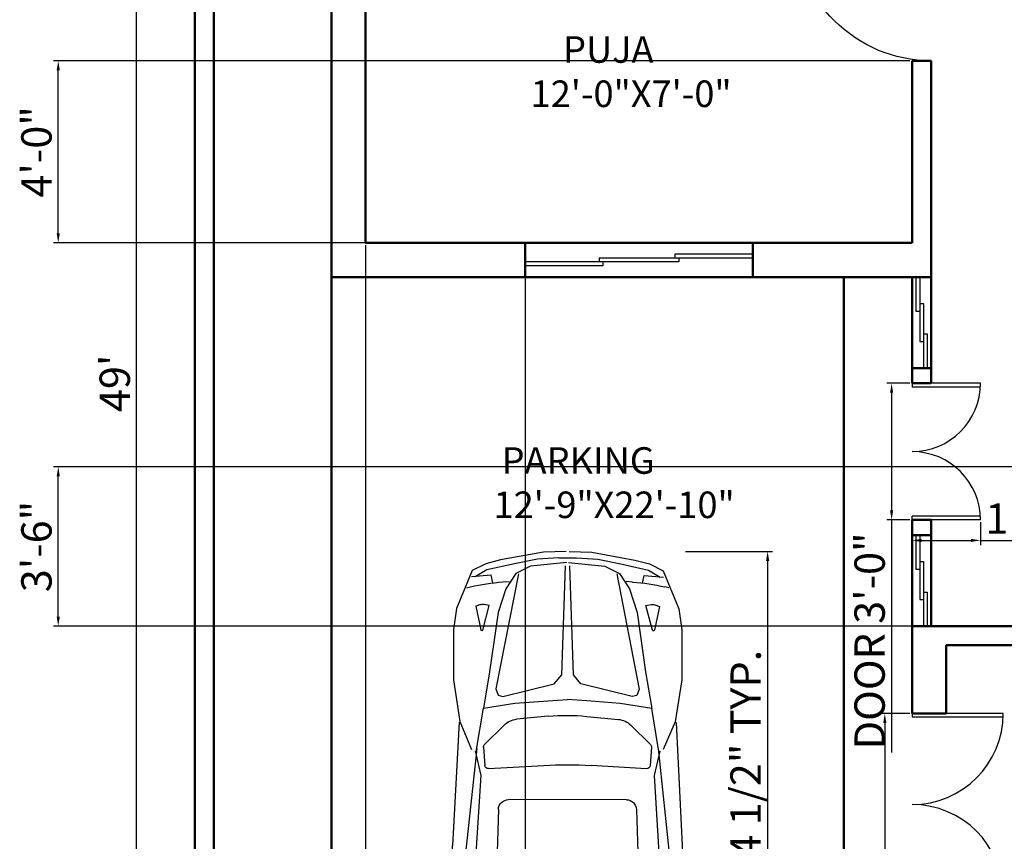
# Model space of a CAD drawing. Units: inches. Extents: x 1913 to 5309, y 1003 to 1733.
# Tile 3 of 23: x 1913 to 2173, y 1272 to 1489. Entities that reach past the tile are written whole.
import ezdxf

# ---------------------------------------------------------------- set-up
doc = ezdxf.new("R2010")
doc.units = ezdxf.units.IN
for name, color, linetype, lineweight in [('A-ANNO-DIMS', 2, 'Continuous', 18), ('A-AREA-IDEN', 3, 'Continuous', 18), ('A-DOOR', 4, 'Continuous', 25), ('A-EQPM', 8, 'Continuous', 18), ('A-GLAZ', 5, 'Continuous', 25), ('A-WALL', 7, 'Continuous', 50)]:
    doc.layers.add(name, color=color, linetype=linetype, lineweight=lineweight)
doc.layers.add('L9012X$0', color=2, linetype='Continuous')
doc.styles.get("Standard").update_dxf_attribs({"font": 'arial.ttf'})
doc.dimstyles.new('ISO-25', dxfattribs={"dimtxt": 8, "dimasz": 2.5, "dimexe": 1.25, "dimexo": 0.625, "dimtad": 1, "dimdec": 1, "dimlunit": 3, "dimtxsty": 'Standard', "dimcen": 2.5, "dimclrd": 256, "dimclrt": 1, "dimadec": 0, "dimazin": 0, "dimtfac": 1, "dimtdec": 1, "dimtmove": 0, "dimatfit": 3, "dimfxl": 1, "dimarcsym": 0})

# ---------------------------------------------------------------- blocks, each defined once
blk = doc.blocks.new("MD D 4'")
for p, q in [((0, 24), (0, 0)), ((1, 24), (1, 0)), ((47, 24), (47, 0)), ((48, 24), (48, 0)), ((0, 0), (1, 0)), ((48, 0), (47, 0))]:
    blk.add_line(p, q)
for centre, start, end in [((0, 0), 0, 90), ((48, 0), 90, 180)]:
    blk.add_arc(centre, 24, start, end)
blk = doc.blocks.new('*D20')
at = {"layer": 'A-ANNO-DIMS', "color": 0, "lineweight": -2, "transparency": 16777216}
for p, q in [((1958.75, 1686.96), (1942.76, 1686.96)), ((1944.01, 1101.46), (1944.01, 1684.46)), ((1958.75, 1098.96), (1942.76, 1098.96))]:
    blk.add_line(p, q, dxfattribs=at)
at = {"layer": 'A-ANNO-DIMS', "color": 0, "transparency": 16777216}
for points in [[(1943.6, 1684.46), (1944.43, 1684.46), (1944.01, 1686.96)], [(1943.6, 1101.46), (1944.43, 1101.46), (1944.01, 1098.96)]]:
    blk.add_solid(points, dxfattribs=at)
at = {"layer": 'Defpoints', "color": 0, "transparency": 16777216}
for p in [(1944.01, 1686.96), (1959.37, 1686.96), (1959.37, 1098.96)]:
    blk.add_point(p, dxfattribs=at)
at = {"layer": 'A-ANNO-DIMS', "color": 0, "transparency": 16777216, "insert": (1939.3, 1392.96), "char_height": 8, "attachment_point": 5, "rotation": 90}
blk.add_mtext("49'", dxfattribs=at)
blk = doc.blocks.new("D1 3'")
for p, q in [((0, 36), (0, 0)), ((1, 36), (1, 0)), ((0, 0), (1, 0))]:
    blk.add_line(p, q)
blk.add_arc((0, 0), 36, 0, 90)
blk = doc.blocks.new('12')
for p, q in [((2191.03, 1363.76), (2191.03, 1345.76)), ((2192.03, 1363.74), (2192.03, 1345.76)), ((2226.03, 1363.74), (2226.03, 1345.76)), ((2227.03, 1363.76), (2227.03, 1345.76)), ((2191.03, 1345.76), (2192.03, 1345.76)), ((2227.03, 1345.76), (2226.03, 1345.76))]:
    blk.add_line(p, q)
for centre, start, end in [((2191.03, 1345.76), 0, 90), ((2227.03, 1345.76), 90, 180)]:
    blk.add_arc(centre, 18, start, end)
blk = doc.blocks.new('A1099DC')
at = {"color": 0, "linetype": 'ByBlock'}
for p, q in [((1279.298465, 804.448389), (2201.430588, 851.890505)), ((2602.736326, 846.078152), (3356.693814, 785.353187)), ((272.228253, 749.073842), (265.114727, 718.465169)), ((1475.52921, 670.226262), (2282.402739, 758.004075)), ((2519.280414, 756.817792), (3387.476361, 653.818028)), ((2851.341839, 715.213377), (3126.60716, 755.701993)), ((3488.458929, 772.663345), (3732.658862, 759.86454)), ((139.051458, 595.027331), (190.951238, 683.213377)), ((179.200345, 564.515703), (190.951238, 709.631982)), ((398.733388, 644.315148), (411.280494, 678.748261)), ((411.280494, 678.748261), (588.616917, 641.417897)), ((1482.852352, 674.283145), (1175.286956, 622.180789)), ((1494.603245, 682.841284), (1678.210958, 641.166865)), ((1678.210958, 641.166865), (2462.684993, 690.847736)), ((2656.476214, 692.831247), (3376.704709, 662.004075)), ((3909.27561, 688.812956), (3837.725727, 693.401722)), ((3867.794139, 700.329656), (3900.059395, 686.767505)), ((3921.162781, 527.618662), (3921.162781, 676.138994)), ((3925.383812, 676.122818), (3955.306409, 663.545364)), ((92.537504, 388.14361), (139.051458, 595.027331)), ((405.405047, 577.538958), (396.874865, 615.894428)), ((589.014326, 626.599587), (405.405047, 577.538958)), ((1300.814287, 466.658131), (1445.712032, 613.104998)), ((1465.665584, 620.56924), (1602.893878, 610.287296)), ((3376.704709, 662.004075), (3510.708679, 626.736433)), ((236.043912, 551.980927), (179.200345, 564.515703)), ((1626.354615, 583.507504), (1602.652901, 169.222264)), ((1933.148906, 509.557888), (2330.980062, 522.200075)), ((3704.596898, 536.993674), (3795.675135, 473.385795)), ((229.117398, 477.634662), (225.714299, 427.957563)), ((2409.60024, 445.938054), (2410.49349, -460.09121)), ((3493.960271, 465.734554), (3507.923021, 209.166865)), ((3522.252709, 492.345257), (3666.066199, 475.644444)), ((3841.786866, 503.451367), (3910.58243, 515.096797)), ((3901.001848, 514.780764), (3957.150905, 375.772812)), ((57.774444, 216.608726), (92.537504, 388.14361)), ((1235.045743, 136.116317), (1257.419842, 373.755108)), ((1860.238743, -448.635916), (1859.369151, 433.397797)), ((3753.293176, 397.789551), (3815.226005, 132.124765)), ((3839.396146, 426.841284), (3888.358202, 417.538958)), ((3857.610793, 379.525702), (3912.067615, 118.157673)), ((3888.358202, 417.538958), (3983.199613, 359.957848)), ((3983.199613, 359.957848), (4035.448301, 43.94997)), ((49.168662, 58.00681), (57.774444, 216.608726)), ((3507.923021, 209.166865), (3507.64153, -4.333678)), ((4019.086894, 150.376168), (4084.69605, 122.469191)), ((4084.69605, 122.469191), (4109.177079, 60.329656)), ((4109.177079, 60.329656), (4113.094043, -5.158716)), ((3508.347273, -221.154823), (3507.644805, -7.65525)), ((3983.920268, -371.008369), (4035.545755, -54.898082)), ((4084.948231, -133.320044), (4109.306686, -71.132359)), ((4109.306686, -71.132359), (4113.094514, -5.636391)), ((49.301278, -76.507426), (58.219773, -235.092064)), ((3754.088875, -409.293325), (3815.497749, -143.506937)), ((3858.370276, -390.823819), (3912.311631, -129.348921)), ((4019.394229, -161.356334), (4084.948231, -133.320044)), ((1235.330373, -152.586046), (1258.173002, -390.180259)), ((1627.520644, -599.204785), (1603.002095, -184.967086)), ((3494.890446, -477.749545), (3508.347273, -221.154823)), ((58.219773, -235.092064), (93.320996, -406.558069)), ((93.320996, -406.558069), (140.24279, -613.349673)), ((3840.248961, -438.175225), (3889.19258, -428.776374)), ((3889.19258, -428.776374), (3983.920268, -371.008369)), ((3902.027941, -525.993061), (3957.902795, -386.874665)), ((230.077082, -495.779641), (226.576036, -446.109349)), ((1301.750547, -482.997536), (1446.936772, -629.158411)), ((3523.2353, -504.304409), (3667.01558, -487.320059)), ((3705.667171, -548.593196), (3796.61981, -484.805853)), ((3842.790735, -514.780444), (3911.609128, -526.290202)), ((237.150178, -570.112104), (180.331436, -582.758939)), ((180.331436, -582.758939), (192.368445, -727.851766)), ((1934.168526, -524.650381), (2332.023837, -536.508105)), ((3922.214148, -538.79118), (3922.506998, -687.311224)), ((140.24279, -613.349673), (192.316354, -701.433212)), ((406.561378, -595.336142), (398.106841, -633.708356)), ((400.0214, -662.125356), (412.636377, -696.533662)), ((590.267037, -644.034637), (406.561378, -595.336142)), ((412.636377, -696.533662), (589.898847, -658.853701)), ((1484.19765, -690.263206), (1176.530118, -638.767405)), ((1466.905004, -636.583294), (1604.112757, -626.030785)), ((1495.965396, -698.798158), (1679.490579, -656.761786)), ((1679.490579, -656.761786), (2464.061049, -704.895745)), ((3378.022114, -674.249887), (3511.956283, -638.718087)), ((273.723073, -767.133288), (266.549207, -736.538701)), ((1476.866524, -686.22077), (2283.911563, -772.40743)), ((2520.786439, -770.754078), (3388.777604, -666.042617)), ((2657.855804, -706.497136), (3378.022114, -674.249887)), ((2852.765183, -728.494989), (3128.109803, -768.440762)), ((3910.644841, -700.0086), (3839.104145, -704.738438)), ((3869.186159, -711.60707), (3901.424611, -697.981326)), ((3926.727989, -687.286725), (3956.625729, -674.650294)), ((2604.418191, -859.849707), (3358.254477, -797.638217)), ((3489.994314, -784.688586), (3734.168535, -771.408296)), ((1280.900818, -820.829563), (2203.124693, -866.453338))]:
    blk.add_line(p, q, dxfattribs=at)
for points in [[(-0.000783, 0.794772), (5.385043, 172.701749), (63.649891, 493.818028), (92.537504, 603.957563), (144.437284, 705.166865), (428.417214, 824.236633), (585.095796, 846.190121), (961.406447, 846.190121), (1274.27399, 797.818028), (1482.852352, 709.631982)], [(83.345007, -3.206171), (111.32237, 268.957533), (164.563706, 379.583828), (279.999271, 453.709838), (456.549665, 511.628518), (901.254996, 574.918954), (1175.286956, 622.180789), (1137.52997, 385.548359), (1118.345181, 137.317882), (1109.829198, -8.358455)], [(168.178729, 359.003083), (1030.214866, 528.397865), (1077.798844, 510.531569), (1086.170082, 475.285426), (992.832238, 91.960378), (924.218938, 35.478085), (108.447994, 6.034416)], [(0.019119, -19.392451), (5.743899, -191.288474), (64.641806, -512.289243), (93.746535, -622.371603), (145.845778, -723.478374), (430.059935, -841.987962), (586.7815, -863.632471), (963.091723, -863.198028), (1275.863278, -814.209121), (1484.26735, -725.611974)], [(83.356858, -15.227176), (111.870816, -287.335185), (165.330179, -397.856284), (280.911681, -471.754535), (457.575935, -529.324983), (902.4055, -592.045995), (1176.530118, -638.767405), (1138.306616, -402.209884), (1118.632407, -154.017717), (1109.829198, -8.358455)], [(168.904615, -377.268451), (1031.273389, -545.270714), (1078.822046, -527.310627), (1087.123771, -492.048047), (993.030273, -108.907787), (924.305735, -52.560894), (108.478017, -24.418246)]]:
    blk.add_lwpolyline(points, dxfattribs=at)
for centre, radius, start, end in [((2358.037832, -2192.08357), 3048, 85.395244, 92.945173), ((2399.99649, 588.663508), 206.166238, 54.649181, 124.776949), ((3392.740754, -1053.630025), 1828.8, 86.999806, 98.367602), ((3718.678317, 475.802507), 284.405862, 57.329946, 87.182375), ((1749.553982, 373.478072), 1524, 166.916578, 176.08111), ((2578.271641, -1134.295865), 1828.8, 87.549126, 93.623712), ((4191.049821, 605.937201), 363.988953, 166.096081, 196.353514), ((3908.462781, 676.138994), 12.7, 0, 86.330429), ((446.46332, 626.922805), 50.8, 159.97873, 192.538409), ((587.047263, 633.961317), 7.62, 284.960009, 78.112462), ((1463.767788, 595.240237), 25.4, 85.715073, 135.304647), ((1600.996082, 584.958293), 25.4, 356.725615, 85.715073), ((3355.555414, 37.211519), 609.6, 55.070043, 75.255062), ((3320.85101, 50.338397), 847.430844, 356.245089, 44.519453), ((3896.252417, 523.051998), 152.4, 46.38363, 67.20138), ((3700.933354, 318.064082), 435.542335, 30.457681, 46.38363), ((2333.400307, 446.03852), 76.2, 359.924458, 91.82012), ((3908.462781, 527.618662), 12.7, 279.607718, 0), ((3204.184594, 25.950693), 1011.814461, 358.069446, 30.457681), ((1409.148822, 359.469565), 152.4, 135.304647, 174.62136), ((1935.569151, 433.396333), 76.2, 91.82012, 179.9989), ((3519.322741, 467.114813), 25.4, 83.37601, 183.115039), ((3654.346327, 374.722669), 101.6, 13.122645, 83.37601), ((3708.414764, 348.440256), 152.4, 11.769371, 55.070043), ((4645.676894, -4.872483), 3048, 176.725615, 183.38736), ((2752.335538, -6.739118), 1524, 174.62136, 185.491615), ((3221.54491, -6.276527), 609.6, 346.99033, 13.122645), ((3315.283499, -6.18411), 609.6, 348.343604, 11.769371), ((1266.577845, -8.050136), 1219.2, 176.894161, 183.218814), ((3734.73098, -5.770579), 304.8, 350.724636, 9.388339), ((3320.962449, -62.69553), 847.430844, 315.593523, 3.867886), ((3204.248172, -38.537915), 1011.814461, 329.655294, 2.043529), ((1409.873518, -375.595566), 152.4, 185.491615, 224.808328), ((3655.096735, -386.42159), 101.6, 276.736965, 346.99033), ((3709.113243, -360.032616), 152.4, 305.042932, 348.343604), ((1750.305335, -388.625277), 1524, 184.031865, 193.196397), ((1936.438592, -448.484202), 76.2, 180.114076, 268.292856), ((2334.293902, -460.341926), 76.2, 268.292856, 0.188517), ((3520.255588, -479.079792), 25.4, 176.997936, 276.736965), ((4192.255091, -616.577407), 363.988953, 163.759461, 194.016894), ((3355.640902, -49.500248), 609.6, 284.857913, 305.042932), ((3909.514173, -538.816222), 12.7, 0.112975, 80.505257), ((3701.571953, -329.671253), 435.542335, 313.729345, 329.655294), ((447.716945, -644.638934), 50.8, 167.574566, 200.134245), ((588.314493, -651.400231), 7.62, 282.000513, 75.152966), ((1464.957267, -611.258083), 25.4, 224.808328, 274.397903), ((1602.165021, -600.705574), 25.4, 274.397903, 3.38736), ((3897.294828, -534.273643), 152.4, 292.911596, 313.729345), ((2576.048678, 1120.472221), 1828.8, 266.489263, 272.563849), ((3719.627907, -487.374382), 284.405862, 272.930601, 302.78303), ((3909.807023, -687.336265), 12.7, 273.782546, 0.112975), ((2401.171182, -602.835323), 206.166238, 235.336026, 305.463794), ((3390.675263, 1041.412497), 1828.8, 261.745373, 273.113169), ((2353.729565, 2177.823616), 3048, 267.167802, 274.717731)]:
    blk.add_arc(centre, radius, start, end, dxfattribs=at)
blk = doc.blocks.new('VI')
at = {"layer": 'L9012X$0'}
blk.add_blockref('A1099DC', (0, 0), dxfattribs=at)
blk = doc.blocks.new('WIN-24')
for p, q in [((0, 15), (0, 24)), ((1, 7), (1, 24)), ((2, 17), (1, 17)), ((2, 0), (2, 17)), ((1, 15), (0, 15)), ((3, 9), (2, 9)), ((3, 0), (3, 9)), ((2, 7), (1, 7))]:
    blk.add_line(p, q)
blk = doc.blocks.new('WIN-60')
for p, q in [((0, 60), (0, 39.5)), ((1, 60), (1, 19.5)), ((0, 39.5), (1, 39.5)), ((1, 40.5), (2, 40.5)), ((2, 40.5), (2, 0)), ((1, 19.5), (2, 19.5)), ((2, 20.5), (3, 20.5)), ((3, 20.5), (3, 0))]:
    blk.add_line(p, q)
blk = doc.blocks.new('*D81')
at = {"layer": 'A-ANNO-DIMS', "color": 0, "lineweight": -2, "transparency": 16777216}
for p, q in [((2147.75, 1305.96), (2139.92, 1305.96)), ((2147.75, 1257.96), (2139.92, 1257.96))]:
    blk.add_line(p, q, dxfattribs=at)
at = {"layer": 'A-ANNO-DIMS', "lineweight": -2, "transparency": 16777216}
for p, q in [((2141.17, 1303.46), (2141.17, 1260.46)), ((2141.17, 1257.96), (2141.17, 1138.14))]:
    blk.add_line(p, q, dxfattribs=at)
at = {"layer": 'A-ANNO-DIMS', "transparency": 16777216}
for points in [[(2140.76, 1303.46), (2141.59, 1303.46), (2141.17, 1305.96)], [(2140.76, 1260.46), (2141.59, 1260.46), (2141.17, 1257.96)]]:
    blk.add_solid(points, dxfattribs=at)
at = {"layer": 'Defpoints', "color": 0, "transparency": 16777216}
for p in [(2148.37, 1305.96), (2141.17, 1257.96), (2148.37, 1257.96)]:
    blk.add_point(p, dxfattribs=at)
at = {"layer": 'A-ANNO-DIMS', "color": 1, "transparency": 16777216, "insert": (2136.41, 1196.8), "char_height": 8, "attachment_point": 5, "rotation": 90}
blk.add_mtext('MAIN DOOR 4\'-0" TYP.', dxfattribs=at)
blk = doc.blocks.new('*D85')
at = {"layer": 'A-ANNO-DIMS', "color": 0, "lineweight": -2, "transparency": 16777216}
for p, q in [((2088.63, 1348.67), (2111.54, 1348.67)), ((2088.63, 1200.09), (2111.54, 1200.09))]:
    blk.add_line(p, q, dxfattribs=at)
at = {"layer": 'A-ANNO-DIMS', "lineweight": -2, "transparency": 16777216}
blk.add_line((2110.29, 1346.17), (2110.29, 1202.59), dxfattribs=at)
at = {"layer": 'A-ANNO-DIMS', "transparency": 16777216}
for points in [[(2109.87, 1346.17), (2110.71, 1346.17), (2110.29, 1348.67)], [(2109.87, 1202.59), (2110.71, 1202.59), (2110.29, 1200.09)]]:
    blk.add_solid(points, dxfattribs=at)
at = {"layer": 'Defpoints', "color": 0, "transparency": 16777216}
for p in [(2088, 1348.67), (2088, 1200.09), (2110.29, 1200.09)]:
    blk.add_point(p, dxfattribs=at)
at = {"layer": 'A-ANNO-DIMS', "color": 1, "transparency": 16777216, "insert": (2105.53, 1274.38), "char_height": 8, "attachment_point": 5, "rotation": 90}
blk.add_mtext('CAR 12\'-4 1/2" TYP.', dxfattribs=at)
blk = doc.blocks.new('*D87')
at = {"layer": 'A-ANNO-DIMS', "color": 0, "lineweight": -2, "transparency": 16777216}
for p, q in [((2147.75, 1392.96), (2141.72, 1392.96)), ((2147.75, 1356.96), (2141.72, 1356.96))]:
    blk.add_line(p, q, dxfattribs=at)
at = {"layer": 'A-ANNO-DIMS', "lineweight": -2, "transparency": 16777216}
for p, q in [((2142.97, 1390.46), (2142.97, 1359.46)), ((2142.97, 1356.96), (2142.97, 1295.71))]:
    blk.add_line(p, q, dxfattribs=at)
at = {"layer": 'A-ANNO-DIMS', "transparency": 16777216}
for points in [[(2142.56, 1390.46), (2143.39, 1390.46), (2142.97, 1392.96)], [(2142.56, 1359.46), (2143.39, 1359.46), (2142.97, 1356.96)]]:
    blk.add_solid(points, dxfattribs=at)
at = {"layer": 'Defpoints', "color": 0, "transparency": 16777216}
for p in [(2148.37, 1392.96), (2142.97, 1356.96), (2148.37, 1356.96)]:
    blk.add_point(p, dxfattribs=at)
at = {"layer": 'A-ANNO-DIMS', "color": 1, "transparency": 16777216, "insert": (2138.21, 1325.09), "char_height": 8, "attachment_point": 5, "rotation": 90}
blk.add_mtext('DOOR 3\'-0"', dxfattribs=at)
blk = doc.blocks.new('*D88')
at = {"layer": 'A-ANNO-DIMS', "color": 0, "lineweight": -2, "transparency": 16777216}
for p, q in [((2148.37, 1356.34), (2148.37, 1350.31)), ((2166.37, 1356.34), (2166.37, 1350.31))]:
    blk.add_line(p, q, dxfattribs=at)
at = {"layer": 'A-ANNO-DIMS', "lineweight": -2, "transparency": 16777216}
for p, q in [((2150.87, 1351.56), (2163.87, 1351.56)), ((2166.37, 1351.56), (2190.64, 1351.56))]:
    blk.add_line(p, q, dxfattribs=at)
at = {"layer": 'A-ANNO-DIMS', "transparency": 16777216}
for points in [[(2150.87, 1351.98), (2150.87, 1351.15), (2148.37, 1351.56)], [(2163.87, 1351.98), (2163.87, 1351.15), (2166.37, 1351.56)]]:
    blk.add_solid(points, dxfattribs=at)
at = {"layer": 'Defpoints', "color": 0, "transparency": 16777216}
for p in [(2148.37, 1356.96), (2166.37, 1356.96), (2166.37, 1351.56)]:
    blk.add_point(p, dxfattribs=at)
at = {"layer": 'A-ANNO-DIMS', "color": 1, "transparency": 16777216, "insert": (2179.75, 1356.27), "char_height": 8, "attachment_point": 5}
blk.add_mtext('1\'-6"', dxfattribs=at)
blk = doc.blocks.new('*D92')
at = {"layer": 'A-ANNO-DIMS', "color": 0, "lineweight": -2, "transparency": 16777216}
for p, q in [((2004.37, 1429.34), (2004.37, 1032.04)), ((2046.37, 1429.34), (2046.37, 1032.04))]:
    blk.add_line(p, q, dxfattribs=at)
at = {"layer": 'A-ANNO-DIMS', "lineweight": -2, "transparency": 16777216}
blk.add_line((2006.87, 1033.29), (2043.87, 1033.29), dxfattribs=at)
at = {"layer": 'A-ANNO-DIMS', "transparency": 16777216}
for points in [[(2006.87, 1033.7), (2006.87, 1032.87), (2004.37, 1033.29)], [(2043.87, 1033.7), (2043.87, 1032.87), (2046.37, 1033.29)]]:
    blk.add_solid(points, dxfattribs=at)
at = {"layer": 'Defpoints', "color": 0, "transparency": 16777216}
for p in [(2004.37, 1429.96), (2046.37, 1429.96), (2046.37, 1033.29)]:
    blk.add_point(p, dxfattribs=at)
at = {"layer": 'A-ANNO-DIMS', "color": 1, "transparency": 16777216, "insert": (2025.37, 1038), "char_height": 8, "attachment_point": 5}
blk.add_mtext('3\'-6"', dxfattribs=at)
blk = doc.blocks.new('*D95')
at = {"layer": 'A-ANNO-DIMS', "color": 0, "lineweight": -2, "transparency": 16777216}
for p, q in [((2147.75, 1477.96), (1922.12, 1477.96)), ((2147.75, 1429.96), (1922.12, 1429.96))]:
    blk.add_line(p, q, dxfattribs=at)
at = {"layer": 'A-ANNO-DIMS', "lineweight": -2, "transparency": 16777216}
blk.add_line((1923.37, 1432.46), (1923.37, 1475.46), dxfattribs=at)
at = {"layer": 'A-ANNO-DIMS', "transparency": 16777216}
for points in [[(1922.96, 1475.46), (1923.79, 1475.46), (1923.37, 1477.96)], [(1922.96, 1432.46), (1923.79, 1432.46), (1923.37, 1429.96)]]:
    blk.add_solid(points, dxfattribs=at)
at = {"layer": 'Defpoints', "color": 0, "transparency": 16777216}
for p in [(1923.37, 1477.96), (2148.37, 1477.96), (2148.37, 1429.96)]:
    blk.add_point(p, dxfattribs=at)
at = {"layer": 'A-ANNO-DIMS', "color": 1, "transparency": 16777216, "insert": (1918.66, 1453.96), "char_height": 8, "attachment_point": 5, "rotation": 90}
blk.add_mtext('4\'-0"', dxfattribs=at)
blk = doc.blocks.new('*D102')
at = {"layer": 'A-ANNO-DIMS', "color": 0, "lineweight": -2, "transparency": 16777216}
for p, q in [((2412.75, 1370.96), (1922.12, 1370.96)), ((2412.75, 1328.96), (1922.12, 1328.96))]:
    blk.add_line(p, q, dxfattribs=at)
at = {"layer": 'A-ANNO-DIMS', "lineweight": -2, "transparency": 16777216}
blk.add_line((1923.37, 1331.46), (1923.37, 1368.46), dxfattribs=at)
at = {"layer": 'A-ANNO-DIMS', "transparency": 16777216}
for points in [[(1922.96, 1368.46), (1923.79, 1368.46), (1923.37, 1370.96)], [(1922.96, 1331.46), (1923.79, 1331.46), (1923.37, 1328.96)]]:
    blk.add_solid(points, dxfattribs=at)
at = {"layer": 'Defpoints', "color": 0, "transparency": 16777216}
for p in [(1923.37, 1370.96), (2413.37, 1370.96), (2413.37, 1328.96)]:
    blk.add_point(p, dxfattribs=at)
at = {"layer": 'A-ANNO-DIMS', "color": 1, "transparency": 16777216, "insert": (1918.66, 1349.96), "char_height": 8, "attachment_point": 5, "rotation": 90}
blk.add_mtext('3\'-6"', dxfattribs=at)

msp = doc.modelspace()

# ---------------------------------------------------------------- linework, layer by layer
at = {"layer": 'A-WALL'}
for p, q in [((1959.37, 1098.96), (1959.37, 1686.96)), ((1995.37, 1686.96), (1995.37, 1420.96)), ((1964.37, 1103.96), (1964.37, 1681.96)), ((2004.37, 1513.96), (2004.37, 1429.96)), ((2148.37, 1477.96), (2148.37, 1429.96)), ((2148.37, 1477.96), (2153.37, 1477.96)), ((2153.37, 1477.96), (2153.37, 1392.96)), ((2004.37, 1429.96), (2148.37, 1429.96)), ((2046.37, 1420.96), (2046.37, 1429.96)), ((2106.37, 1420.96), (2106.37, 1429.96)), ((1995.37, 1420.96), (2153.37, 1420.96)), ((1995.37, 1420.96), (1995.37, 1146.96)), ((2130.37, 1420.96), (2130.37, 1257.96)), ((2148.37, 1420.96), (2148.37, 1392.96)), ((2148.37, 1396.96), (2153.37, 1396.96)), ((2148.37, 1392.96), (2153.37, 1392.96)), ((2148.37, 1356.96), (2153.37, 1356.96)), ((2148.37, 1356.96), (2148.37, 1305.96)), ((2153.37, 1356.96), (2153.37, 1328.96)), ((2148.37, 1352.96), (2153.37, 1352.96)), ((2148.37, 1328.96), (2281.37, 1328.96)), ((2157.37, 1323.96), (2281.37, 1323.96)), ((2157.37, 1323.96), (2157.37, 1305.96)), ((2148.37, 1305.96), (2157.37, 1305.96))]:
    msp.add_line(p, q, dxfattribs=at)

# ---------------------------------------------------------------- block references
at = {"layer": 'A-DOOR', "xscale": -1, "rotation": 90}
msp.add_blockref("D1 3'", (2153.37, 1513.96), dxfattribs=at)
at = {"layer": 'A-DOOR', "rotation": 270}
for name, p in [('12', (802.61, 3583.99)), ("MD D 4'", (2148.37, 1305.96))]:
    msp.add_blockref(name, p, dxfattribs=at)
at = {"layer": 'A-EQPM', "xscale": -0.0351896714874634, "yscale": 0.0351896714874634, "zscale": 0.0351896714874634, "rotation": 90}
msp.add_blockref('VI', (2057.28, 1348.67), dxfattribs=at)
at = {"layer": 'A-GLAZ'}
for name, p, rotation in [('WIN-60', (2046.37, 1426.96), 270.0000000000014), ('WIN-24', (2152.37, 1420.96), 180), ('WIN-24', (2152.37, 1352.96), 180)]:
    msp.add_blockref(name, p, dxfattribs=dict(at, rotation=rotation))

# ---------------------------------------------------------------- texts
at = {"layer": 'A-AREA-IDEN', "char_height": 7, "attachment_point": 1}
for s, insert in [('    PUJA\\P12\'-0"X7\'-0"', (2047.84, 1484.43)), (' PARKING\\P12\'-9"X22\'-10"', (2038.06, 1376.11))]:
    msp.add_mtext_dynamic_manual_height_columns(s, width=86.9528, gutter_width=12.5, heights=[0], dxfattribs=dict(at, insert=insert))

# ---------------------------------------------------------------- dimensions: what is measured, and where the dimension line sits
at = {"layer": 'A-ANNO-DIMS'}
for base, p1, p2, override, picture, middle in [((1944.01, 1686.96), (1959.37, 1098.96), (1959.37, 1686.96), {"dimclrd": 0, "dimclre": 0, "dimclrt": 0}, '*D20', (1939.3, 1392.96)), ((1923.37, 1477.96), (2148.37, 1429.96), (2148.37, 1477.96), {"dimdec": 1, "dimlfac": 1, "dimrnd": 0, "dimzin": 1, "dimdsep": 46, "dimlunit": 4, "dimfrac": 2}, '*D95', (1918.66, 1453.96)), ((1923.37, 1370.96), (2413.37, 1328.96), (2413.37, 1370.96), {"dimdec": 1, "dimlfac": 1, "dimrnd": 0, "dimzin": 1, "dimdsep": 46, "dimlunit": 4, "dimfrac": 2}, '*D102', (1918.66, 1349.96))]:
    dim = msp.add_linear_dim(base=base, p1=p1, p2=p2, angle=90, dimstyle='ISO-25', override=override, dxfattribs=at)
    dim.commit()
    dim.dimension.update_dxf_attribs({"geometry": picture, "text_midpoint": middle})
for base, p1, p2, override, picture, middle in [((2046.37, 1033.29), (2004.37, 1429.96), (2046.37, 1429.96), {"dimdec": 1, "dimlfac": 1, "dimrnd": 0, "dimzin": 1, "dimdsep": 46, "dimlunit": 4, "dimfrac": 2}, '*D92', (2025.37, 1038)), ((2166.37, 1351.56), (2148.37, 1356.96), (2166.37, 1356.96), {"dimdec": 1, "dimrnd": 0, "dimzin": 1, "dimlunit": 4, "dimfrac": 2}, '*D88', (2179.75, 1356.27))]:
    dim = msp.add_linear_dim(base=base, p1=p1, p2=p2, dimstyle='ISO-25', override=override, dxfattribs=at)
    dim.commit()
    dim.dimension.update_dxf_attribs({"geometry": picture, "text_midpoint": middle})
for base, p1, p2, text, picture, middle in [((2142.97, 1356.96), (2148.37, 1392.96), (2148.37, 1356.96), 'DOOR <>', '*D87', (2138.21, 1325.09)), ((2110.29, 1200.09), (2088, 1348.67), (2088, 1200.09), 'CAR <> TYP.', '*D85', (2105.53, 1274.38)), ((2141.17, 1257.96), (2148.37, 1305.96), (2148.37, 1257.96), 'MAIN DOOR <> TYP.', '*D81', (2136.41, 1196.8))]:
    dim = msp.add_linear_dim(base=base, p1=p1, p2=p2, angle=270, text=text, dimstyle='ISO-25', override={"dimdec": 1, "dimrnd": 0, "dimzin": 1, "dimlunit": 4, "dimfrac": 2}, dxfattribs=at)
    dim.commit()
    dim.dimension.update_dxf_attribs({"geometry": picture, "text_midpoint": middle})

doc.saveas('drawing.dxf')
